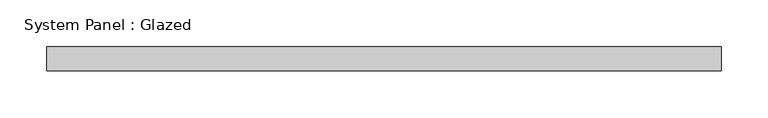
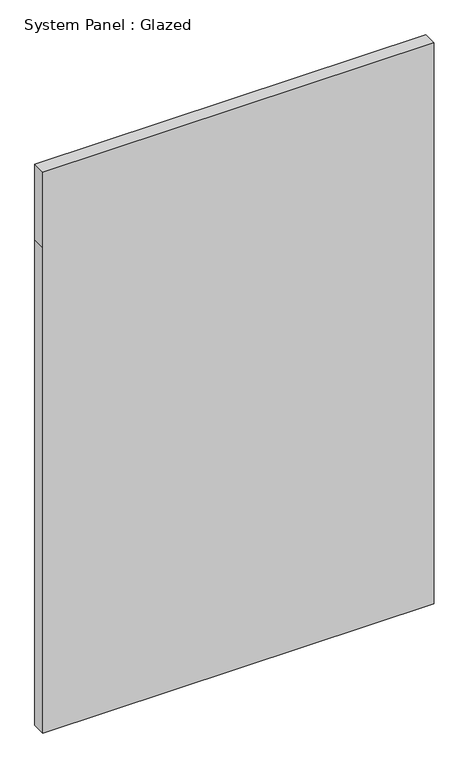
"""IFC4 building model written with IfcOpenShell, lengths in millimetres: plate geometry, System Panel : Glazed."""

from ifc_helpers import new_model, si_unit, frame, origin, place, context, project, spatial, polyline, outline, extrude, source, transform, mapped, element, save


def system_panel_glazed_4fbea3b4(model_context):
    return source(origin(), model_context, "Body", "SweptSolid", [
        extrude(outline(polyline([(0.0, -358.775), (0.0, 358.775), (941.116916, 358.775), (1087.166916, 358.775), (1087.166916, -358.775), (941.116916, -358.775), (0.0, -358.775)])), frame((0.0, 19.05, 0.0), z_axis=(0.0, 1.0, 0.0), x_axis=(0.0, 0.0, 1.0)), (0.0, 0.0, 1.0), 25.4),
    ])


if __name__ == "__main__":
    model = new_model("IFC4")
    model_context = context("Model", 3, world=origin())
    ifc_project = project(units=[si_unit("LENGTHUNIT", "METRE", prefix="MILLI")], contexts=[model_context])
    site = spatial("IfcSite", under=ifc_project)
    building = spatial("IfcBuilding", under=site)
    placement = place(None, origin())
    system_panel_glazed_shape = system_panel_glazed_4fbea3b4(model_context)
    element("IfcPlate", 1, ObjectType="System Panel : Glazed", at=placement, inside=building, context=model_context, shape_type="MappedRepresentation", body=[
        mapped(system_panel_glazed_shape, transform((0.0, 0.0, 0.0), x_axis=(1.0, 0.0, 0.0), y_axis=(0.0, 1.0, 0.0), z_axis=(0.0, 0.0, 1.0))),
    ])
    save(model, "model.ifc")

# Revit data of these elements
# Type "System Panel : Glazed"
#   Construction Type Id = "GSP4R"
#   Analytic Construction = "1/8 in Pilkington single glazing"
#   Visual Light Transmittance = 0.9
#   Solar Heat Gain Coefficient = 0.86
#   Heat Transfer Coefficient (U) = 1.18115 BTU/(h·ft²·°F)
#   Define Thermal Properties by = 1
# Element 1 (IfcPlate, "System Panel : Glazed")
#   Materials on its faces: "Glass"
# Materials
#   "Glass": class "Glass", colour RGB 0 128 192, transparency 0.75, Description = "Soda Lime Glass", Cost = 0
